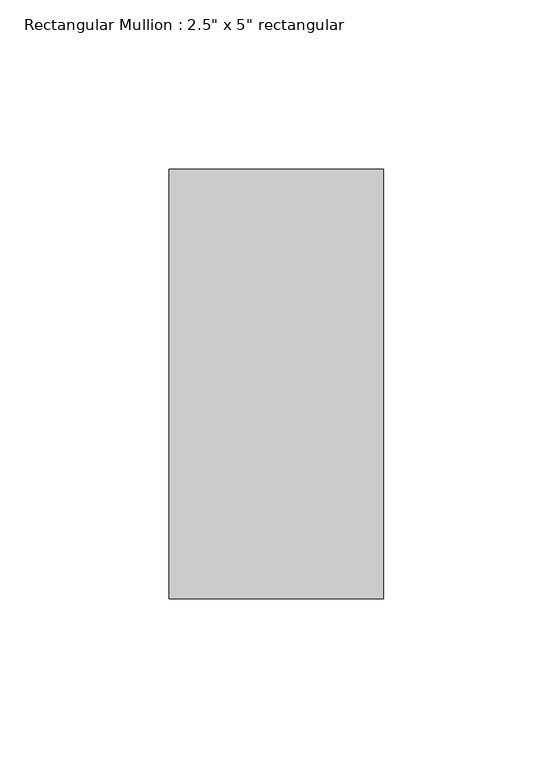
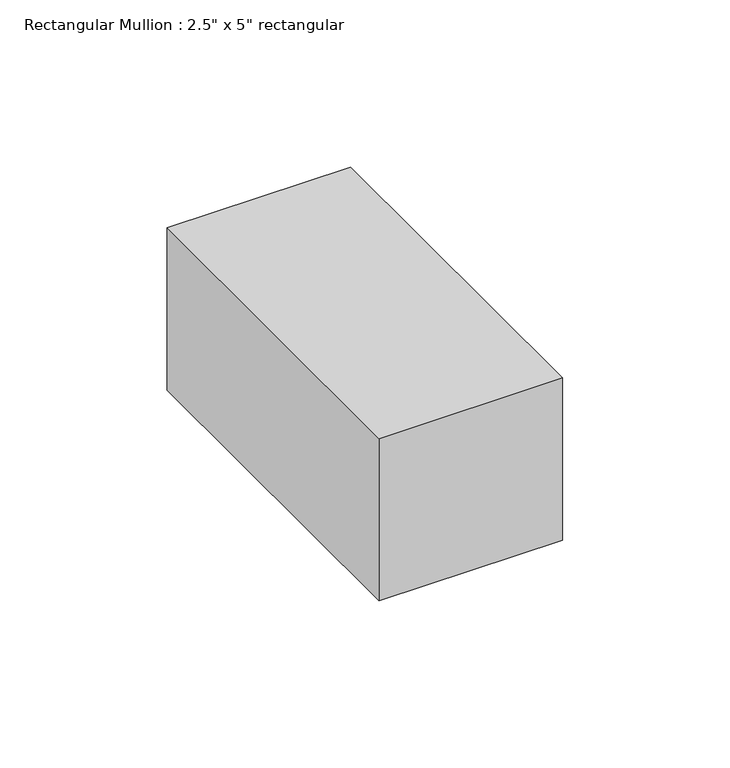
"""IFC4 building model written with IfcOpenShell, lengths in millimetres: member geometry."""

from ifc_helpers import new_model, si_unit, frame, origin, place, context, project, spatial, polyline, outline, extrude, source, transform, mapped, element, save


def member_702056ca(model_context):
    return source(origin(), model_context, "Body", "SweptSolid", [
        extrude(outline(polyline([(0.0, 63.5), (0.0, -63.5), (-63.5, -63.5), (-63.5, 63.5), (0.0, 63.5)])), frame((0.0, 0.0, -59.2666667), z_axis=(0.0, 0.0, 1.0), x_axis=(1.0, 0.0, 0.0)), (0.0, 0.0, 1.0), 59.2666667),
    ])


if __name__ == "__main__":
    model = new_model("IFC4")
    model_context = context("Model", 3, world=origin())
    ifc_project = project(units=[si_unit("LENGTHUNIT", "METRE", prefix="MILLI")], contexts=[model_context])
    site = spatial("IfcSite", under=ifc_project)
    building = spatial("IfcBuilding", under=site)
    placement = place(None, origin())
    member_shape = member_702056ca(model_context)
    element("IfcMember", 1, ObjectType="Rectangular Mullion : 2.5\" x 5\" rectangular", at=placement, inside=building, context=model_context, shape_type="MappedRepresentation", body=[
        mapped(member_shape, transform((0.0, 0.0, 0.0), x_axis=(1.0, 0.0, 0.0), y_axis=(0.0, 1.0, 0.0), z_axis=(0.0, 0.0, 1.0))),
    ])
    save(model, "model.ifc")

# Revit data of these elements
# Type "Rectangular Mullion : 2.5\" x 5\" rectangular"
#   built-in parameter 1007304 = 0.416667 (stored number, unit not read)
#   built-in parameter 1007301 = 0.104167 (stored number, unit not read)
#   built-in parameter 1007300 = 0.104167 (stored number, unit not read)
# Element 1 (IfcMember, "Rectangular Mullion : 2.5\" x 5\" rectangular")
#   Materials on its faces: "Aluminum"
# Materials
#   "Aluminum": class "Metal", colour RGB 247 247 247, transparency 0, Description = "Aluminum 6061", Cost = 0
